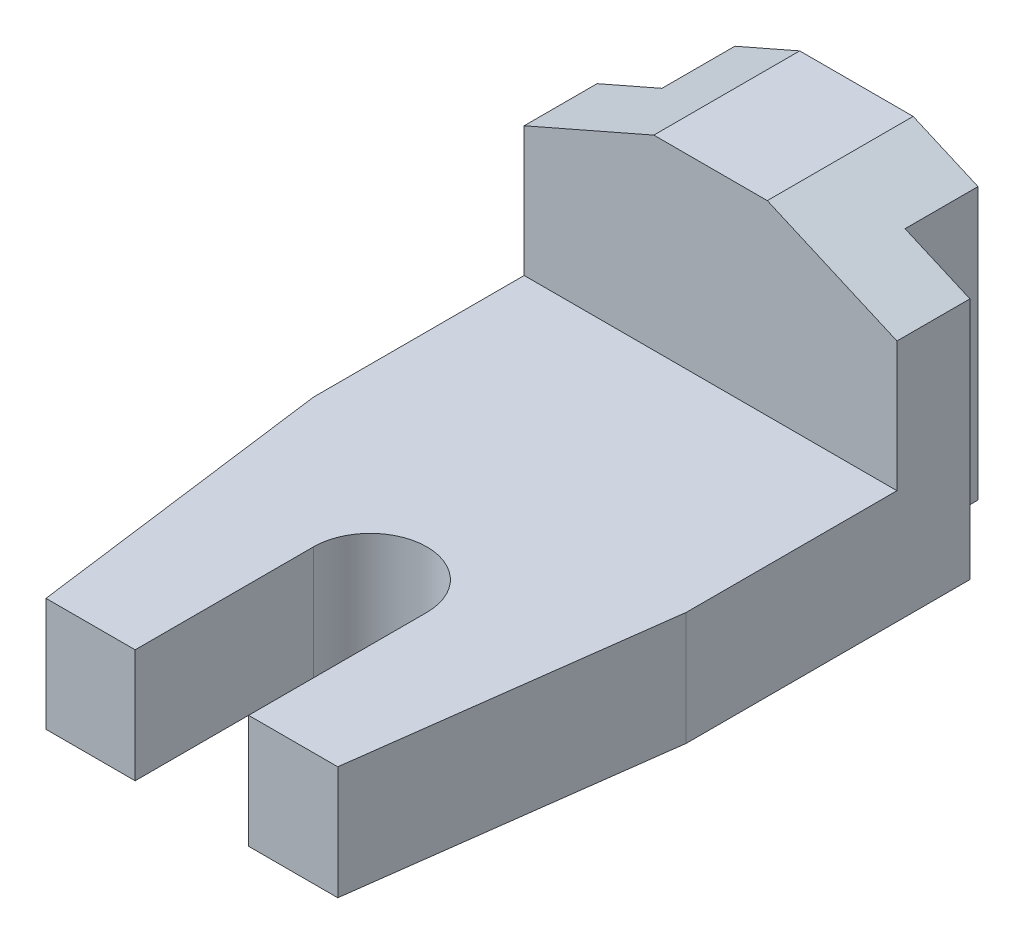
ISO-10303-21;
HEADER;
FILE_DESCRIPTION(('STEP AP214'),'2;1');
FILE_NAME('part.step','',(''),(''),'','','');
FILE_SCHEMA(('AUTOMOTIVE_DESIGN { 1 0 10303 214 1 1 1 1 }'));
ENDSEC;
DATA;
#1=APPLICATION_CONTEXT('core data for automotive mechanical design processes');
#2=APPLICATION_PROTOCOL_DEFINITION('international standard','automotive_design',2000,#1);
#3=PRODUCT_CONTEXT('',#1,'mechanical');
#4=PRODUCT('Part','Part','',(#3));
#5=PRODUCT_RELATED_PRODUCT_CATEGORY('part','',(#4));
#6=PRODUCT_DEFINITION_FORMATION('','',#4);
#7=PRODUCT_DEFINITION_CONTEXT('part definition',#1,'design');
#8=PRODUCT_DEFINITION('design','',#6,#7);
#9=PRODUCT_DEFINITION_SHAPE('','',#8);
#10=(LENGTH_UNIT() NAMED_UNIT(*) SI_UNIT(.MILLI.,.METRE.));
#11=(NAMED_UNIT(*) PLANE_ANGLE_UNIT() SI_UNIT($,.RADIAN.));
#12=(NAMED_UNIT(*) SI_UNIT($,.STERADIAN.) SOLID_ANGLE_UNIT());
#13=UNCERTAINTY_MEASURE_WITH_UNIT(LENGTH_MEASURE(1.E-05),#10,'distance_accuracy_value','');
#14=(GEOMETRIC_REPRESENTATION_CONTEXT(3) GLOBAL_UNCERTAINTY_ASSIGNED_CONTEXT((#13)) GLOBAL_UNIT_ASSIGNED_CONTEXT((#10,
#11,#12)) REPRESENTATION_CONTEXT('',''));
#15=CARTESIAN_POINT('',(0.,0.,0.));
#16=DIRECTION('',(0.,0.,1.));
#17=DIRECTION('',(1.,0.,0.));
#18=AXIS2_PLACEMENT_3D('',#15,#16,#17);
#19=CARTESIAN_POINT('',(-23.,-15.,18.));
#20=DIRECTION('',(1.,0.,0.));
#21=DIRECTION('',(0.,0.,-1.));
#22=AXIS2_PLACEMENT_3D('',#19,#20,#21);
#23=PLANE('',#22);
#24=DIRECTION('',(0.,-1.,0.));
#25=VECTOR('',#24,1.);
#26=CARTESIAN_POINT('',(-23.,22.,9.));
#27=LINE('',#26,#25);
#28=CARTESIAN_POINT('',(-23.,15.,9.));
#29=VERTEX_POINT('',#28);
#30=CARTESIAN_POINT('',(-23.,-15.,9.));
#31=VERTEX_POINT('',#30);
#32=EDGE_CURVE('E332',#29,#31,#27,.T.);
#33=ORIENTED_EDGE('',*,*,#32,.T.);
#34=DIRECTION('',(0.,0.,-1.));
#35=VECTOR('',#34,1.);
#36=CARTESIAN_POINT('',(-23.,-15.,18.));
#37=LINE('',#36,#35);
#38=CARTESIAN_POINT('',(-23.,-15.,44.));
#39=VERTEX_POINT('',#38);
#40=EDGE_CURVE('E207',#39,#31,#37,.T.);
#41=ORIENTED_EDGE('',*,*,#40,.F.);
#42=DIRECTION('',(0.,-1.,0.));
#43=VECTOR('',#42,1.);
#44=CARTESIAN_POINT('',(-23.,-0.999999999999997,44.));
#45=LINE('',#44,#43);
#46=CARTESIAN_POINT('',(-23.,-0.999999999999997,44.));
#47=VERTEX_POINT('',#46);
#48=EDGE_CURVE('E177',#47,#39,#45,.T.);
#49=ORIENTED_EDGE('',*,*,#48,.F.);
#50=DIRECTION('',(0.,0.,-1.));
#51=VECTOR('',#50,1.);
#52=CARTESIAN_POINT('',(-23.,-0.999999999999997,18.));
#53=LINE('',#52,#51);
#54=CARTESIAN_POINT('',(-23.,-0.999999999999997,18.));
#55=VERTEX_POINT('',#54);
#56=EDGE_CURVE('E270',#47,#55,#53,.T.);
#57=ORIENTED_EDGE('',*,*,#56,.T.);
#58=DIRECTION('',(0.,-1.,0.));
#59=VECTOR('',#58,1.);
#60=CARTESIAN_POINT('',(-23.,-15.,18.));
#61=LINE('',#60,#59);
#62=CARTESIAN_POINT('',(-23.,15.,18.));
#63=VERTEX_POINT('',#62);
#64=EDGE_CURVE('E193',#63,#55,#61,.T.);
#65=ORIENTED_EDGE('',*,*,#64,.F.);
#66=DIRECTION('',(0.,0.,-1.));
#67=VECTOR('',#66,1.);
#68=CARTESIAN_POINT('',(-23.,15.,18.));
#69=LINE('',#68,#67);
#70=EDGE_CURVE('E192',#63,#29,#69,.T.);
#71=ORIENTED_EDGE('',*,*,#70,.T.);
#72=EDGE_LOOP('',(#33,#41,#49,#57,#65,#71));
#73=FACE_BOUND('',#72,.T.);
#74=ADVANCED_FACE('F39',(#73),#23,.F.);
#75=CARTESIAN_POINT('',(23.,-15.,18.));
#76=DIRECTION('',(0.,1.,0.));
#77=DIRECTION('',(-1.,0.,0.));
#78=AXIS2_PLACEMENT_3D('',#75,#76,#77);
#79=PLANE('',#78);
#80=DIRECTION('',(1.,0.,0.));
#81=VECTOR('',#80,1.);
#82=CARTESIAN_POINT('',(-23.,-15.,9.));
#83=LINE('',#82,#81);
#84=CARTESIAN_POINT('',(-15.,-15.,9.));
#85=VERTEX_POINT('',#84);
#86=EDGE_CURVE('E174',#31,#85,#83,.T.);
#87=ORIENTED_EDGE('',*,*,#86,.T.);
#88=DIRECTION('',(0.,0.,-1.));
#89=VECTOR('',#88,1.);
#90=CARTESIAN_POINT('',(-15.,-15.,0.));
#91=LINE('',#90,#89);
#92=CARTESIAN_POINT('',(-15.,-15.,0.));
#93=VERTEX_POINT('',#92);
#94=EDGE_CURVE('E163',#85,#93,#91,.T.);
#95=ORIENTED_EDGE('',*,*,#94,.T.);
#96=DIRECTION('',(1.,0.,0.));
#97=VECTOR('',#96,1.);
#98=CARTESIAN_POINT('',(23.,-15.,0.));
#99=LINE('',#98,#97);
#100=CARTESIAN_POINT('',(15.,-15.,0.));
#101=VERTEX_POINT('',#100);
#102=EDGE_CURVE('E63',#93,#101,#99,.T.);
#103=ORIENTED_EDGE('',*,*,#102,.T.);
#104=DIRECTION('',(0.,0.,-1.));
#105=VECTOR('',#104,1.);
#106=CARTESIAN_POINT('',(15.,-15.,0.));
#107=LINE('',#106,#105);
#108=CARTESIAN_POINT('',(15.,-15.,9.));
#109=VERTEX_POINT('',#108);
#110=EDGE_CURVE('E231',#109,#101,#107,.T.);
#111=ORIENTED_EDGE('',*,*,#110,.F.);
#112=DIRECTION('',(-1.,0.,0.));
#113=VECTOR('',#112,1.);
#114=CARTESIAN_POINT('',(23.,-15.,9.));
#115=LINE('',#114,#113);
#116=CARTESIAN_POINT('',(23.,-15.,9.));
#117=VERTEX_POINT('',#116);
#118=EDGE_CURVE('E232',#117,#109,#115,.T.);
#119=ORIENTED_EDGE('',*,*,#118,.F.);
#120=DIRECTION('',(0.,0.,-1.));
#121=VECTOR('',#120,1.);
#122=CARTESIAN_POINT('',(23.,-15.,18.));
#123=LINE('',#122,#121);
#124=CARTESIAN_POINT('',(23.,-15.,44.));
#125=VERTEX_POINT('',#124);
#126=EDGE_CURVE('E206',#125,#117,#123,.T.);
#127=ORIENTED_EDGE('',*,*,#126,.F.);
#128=DIRECTION('',(-0.130454512571387,0.,0.991454295542544));
#129=VECTOR('',#128,1.);
#130=CARTESIAN_POINT('',(23.,-15.,44.));
#131=LINE('',#130,#129);
#132=CARTESIAN_POINT('',(18.,-15.,82.));
#133=VERTEX_POINT('',#132);
#134=EDGE_CURVE('E236',#125,#133,#131,.T.);
#135=ORIENTED_EDGE('',*,*,#134,.T.);
#136=DIRECTION('',(-1.,0.,0.));
#137=VECTOR('',#136,1.);
#138=CARTESIAN_POINT('',(18.,-15.,82.));
#139=LINE('',#138,#137);
#140=CARTESIAN_POINT('',(6.99999999999999,-15.,82.));
#141=VERTEX_POINT('',#140);
#142=EDGE_CURVE('E272',#133,#141,#139,.T.);
#143=ORIENTED_EDGE('',*,*,#142,.T.);
#144=DIRECTION('',(0.,0.,-1.));
#145=VECTOR('',#144,1.);
#146=CARTESIAN_POINT('',(6.99999999999999,-15.,82.));
#147=LINE('',#146,#145);
#148=CARTESIAN_POINT('',(6.99999999999999,-15.,60.));
#149=VERTEX_POINT('',#148);
#150=EDGE_CURVE('E277',#141,#149,#147,.T.);
#151=ORIENTED_EDGE('',*,*,#150,.T.);
#152=CARTESIAN_POINT('',(0.,-15.,60.));
#153=DIRECTION('',(0.,1.,0.));
#154=DIRECTION('',(1.,0.,0.));
#155=AXIS2_PLACEMENT_3D('',#152,#153,#154);
#156=CIRCLE('',#155,7.);
#157=CARTESIAN_POINT('',(-6.99999999999999,-15.,60.));
#158=VERTEX_POINT('',#157);
#159=EDGE_CURVE('E276',#149,#158,#156,.T.);
#160=ORIENTED_EDGE('',*,*,#159,.T.);
#161=DIRECTION('',(0.,0.,1.));
#162=VECTOR('',#161,1.);
#163=CARTESIAN_POINT('',(-7.00000000000001,-15.,82.));
#164=LINE('',#163,#162);
#165=CARTESIAN_POINT('',(-7.00000000000001,-15.,82.));
#166=VERTEX_POINT('',#165);
#167=EDGE_CURVE('E284',#158,#166,#164,.T.);
#168=ORIENTED_EDGE('',*,*,#167,.T.);
#169=DIRECTION('',(-1.,0.,0.));
#170=VECTOR('',#169,1.);
#171=CARTESIAN_POINT('',(-18.,-15.,82.));
#172=LINE('',#171,#170);
#173=CARTESIAN_POINT('',(-18.,-15.,82.));
#174=VERTEX_POINT('',#173);
#175=EDGE_CURVE('E281',#166,#174,#172,.T.);
#176=ORIENTED_EDGE('',*,*,#175,.T.);
#177=DIRECTION('',(-0.130454512571387,0.,-0.991454295542544));
#178=VECTOR('',#177,1.);
#179=CARTESIAN_POINT('',(-23.,-15.,44.));
#180=LINE('',#179,#178);
#181=EDGE_CURVE('E242',#174,#39,#180,.T.);
#182=ORIENTED_EDGE('',*,*,#181,.T.);
#183=ORIENTED_EDGE('',*,*,#40,.T.);
#184=EDGE_LOOP('',(#87,#95,#103,#111,#119,#127,#135,#143,#151,#160,#168,#176,#182,#183));
#185=FACE_BOUND('',#184,.T.);
#186=ADVANCED_FACE('F168',(#185),#79,.F.);
#187=CARTESIAN_POINT('',(-23.,15.,18.));
#188=DIRECTION('',(0.400818834019708,-0.916157334902189,0.));
#189=DIRECTION('',(0.916157334902189,0.400818834019708,0.));
#190=AXIS2_PLACEMENT_3D('',#187,#188,#189);
#191=PLANE('',#190);
#192=DIRECTION('',(0.916157334902189,0.400818834019708,0.));
#193=VECTOR('',#192,1.);
#194=CARTESIAN_POINT('',(-23.,15.,9.));
#195=LINE('',#194,#193);
#196=CARTESIAN_POINT('',(-15.,18.5,9.));
#197=VERTEX_POINT('',#196);
#198=EDGE_CURVE('E11',#29,#197,#195,.T.);
#199=ORIENTED_EDGE('',*,*,#198,.F.);
#200=ORIENTED_EDGE('',*,*,#70,.F.);
#201=DIRECTION('',(-0.916157334902189,-0.400818834019708,0.));
#202=VECTOR('',#201,1.);
#203=CARTESIAN_POINT('',(-23.,15.,18.));
#204=LINE('',#203,#202);
#205=CARTESIAN_POINT('',(-7.,22.,18.));
#206=VERTEX_POINT('',#205);
#207=EDGE_CURVE('E189',#206,#63,#204,.T.);
#208=ORIENTED_EDGE('',*,*,#207,.F.);
#209=DIRECTION('',(0.,0.,-1.));
#210=VECTOR('',#209,1.);
#211=CARTESIAN_POINT('',(-7.,22.,18.));
#212=LINE('',#211,#210);
#213=CARTESIAN_POINT('',(-7.,22.,0.));
#214=VERTEX_POINT('',#213);
#215=EDGE_CURVE('E197',#206,#214,#212,.T.);
#216=ORIENTED_EDGE('',*,*,#215,.T.);
#217=DIRECTION('',(-0.916157334902189,-0.400818834019708,0.));
#218=VECTOR('',#217,1.);
#219=CARTESIAN_POINT('',(-23.,15.,0.));
#220=LINE('',#219,#218);
#221=CARTESIAN_POINT('',(-15.,18.5,0.));
#222=VERTEX_POINT('',#221);
#223=EDGE_CURVE('E191',#214,#222,#220,.T.);
#224=ORIENTED_EDGE('',*,*,#223,.T.);
#225=DIRECTION('',(0.,0.,-1.));
#226=VECTOR('',#225,1.);
#227=CARTESIAN_POINT('',(-15.,18.5,18.));
#228=LINE('',#227,#226);
#229=EDGE_CURVE('E52',#197,#222,#228,.T.);
#230=ORIENTED_EDGE('',*,*,#229,.F.);
#231=EDGE_LOOP('',(#199,#200,#208,#216,#224,#230));
#232=FACE_BOUND('',#231,.T.);
#233=ADVANCED_FACE('F320',(#232),#191,.F.);
#234=CARTESIAN_POINT('',(0.,0.,0.));
#235=DIRECTION('',(0.,0.,-1.));
#236=DIRECTION('',(-1.,0.,0.));
#237=AXIS2_PLACEMENT_3D('',#234,#235,#236);
#238=PLANE('',#237);
#239=ORIENTED_EDGE('',*,*,#102,.F.);
#240=DIRECTION('',(0.,1.,0.));
#241=VECTOR('',#240,1.);
#242=CARTESIAN_POINT('',(-15.,0.,0.));
#243=LINE('',#242,#241);
#244=EDGE_CURVE('E46',#93,#222,#243,.T.);
#245=ORIENTED_EDGE('',*,*,#244,.T.);
#246=ORIENTED_EDGE('',*,*,#223,.F.);
#247=DIRECTION('',(-1.,0.,0.));
#248=VECTOR('',#247,1.);
#249=CARTESIAN_POINT('',(-7.,22.,0.));
#250=LINE('',#249,#248);
#251=CARTESIAN_POINT('',(7.,22.,0.));
#252=VERTEX_POINT('',#251);
#253=EDGE_CURVE('E182',#252,#214,#250,.T.);
#254=ORIENTED_EDGE('',*,*,#253,.F.);
#255=DIRECTION('',(-0.916157334902189,0.400818834019708,0.));
#256=VECTOR('',#255,1.);
#257=CARTESIAN_POINT('',(7.,22.,0.));
#258=LINE('',#257,#256);
#259=CARTESIAN_POINT('',(15.,18.5,0.));
#260=VERTEX_POINT('',#259);
#261=EDGE_CURVE('E178',#260,#252,#258,.T.);
#262=ORIENTED_EDGE('',*,*,#261,.F.);
#263=DIRECTION('',(0.,1.,0.));
#264=VECTOR('',#263,1.);
#265=CARTESIAN_POINT('',(15.,0.,0.));
#266=LINE('',#265,#264);
#267=EDGE_CURVE('E180',#101,#260,#266,.T.);
#268=ORIENTED_EDGE('',*,*,#267,.F.);
#269=EDGE_LOOP('',(#239,#245,#246,#254,#262,#268));
#270=FACE_BOUND('',#269,.T.);
#271=ADVANCED_FACE('F171',(#270),#238,.T.);
#272=CARTESIAN_POINT('',(23.,-15.,18.));
#273=DIRECTION('',(-1.,0.,0.));
#274=DIRECTION('',(0.,0.,1.));
#275=AXIS2_PLACEMENT_3D('',#272,#273,#274);
#276=PLANE('',#275);
#277=ORIENTED_EDGE('',*,*,#126,.T.);
#278=DIRECTION('',(0.,-1.,0.));
#279=VECTOR('',#278,1.);
#280=CARTESIAN_POINT('',(23.,22.,9.));
#281=LINE('',#280,#279);
#282=CARTESIAN_POINT('',(23.,15.,9.));
#283=VERTEX_POINT('',#282);
#284=EDGE_CURVE('E221',#283,#117,#281,.T.);
#285=ORIENTED_EDGE('',*,*,#284,.F.);
#286=DIRECTION('',(0.,0.,-1.));
#287=VECTOR('',#286,1.);
#288=CARTESIAN_POINT('',(23.,15.,18.));
#289=LINE('',#288,#287);
#290=CARTESIAN_POINT('',(23.,15.,18.));
#291=VERTEX_POINT('',#290);
#292=EDGE_CURVE('E201',#291,#283,#289,.T.);
#293=ORIENTED_EDGE('',*,*,#292,.F.);
#294=DIRECTION('',(0.,1.,0.));
#295=VECTOR('',#294,1.);
#296=CARTESIAN_POINT('',(23.,-15.,18.));
#297=LINE('',#296,#295);
#298=CARTESIAN_POINT('',(23.,-0.999999999999996,18.));
#299=VERTEX_POINT('',#298);
#300=EDGE_CURVE('E302',#299,#291,#297,.T.);
#301=ORIENTED_EDGE('',*,*,#300,.F.);
#302=DIRECTION('',(0.,0.,1.));
#303=VECTOR('',#302,1.);
#304=CARTESIAN_POINT('',(23.,-0.999999999999994,18.));
#305=LINE('',#304,#303);
#306=CARTESIAN_POINT('',(23.,-0.999999999999994,44.));
#307=VERTEX_POINT('',#306);
#308=EDGE_CURVE('E244',#299,#307,#305,.T.);
#309=ORIENTED_EDGE('',*,*,#308,.T.);
#310=DIRECTION('',(0.,-1.,0.));
#311=VECTOR('',#310,1.);
#312=CARTESIAN_POINT('',(23.,-0.999999999999994,44.));
#313=LINE('',#312,#311);
#314=EDGE_CURVE('E269',#307,#125,#313,.T.);
#315=ORIENTED_EDGE('',*,*,#314,.T.);
#316=EDGE_LOOP('',(#277,#285,#293,#301,#309,#315));
#317=FACE_BOUND('',#316,.T.);
#318=ADVANCED_FACE('F227',(#317),#276,.F.);
#319=CARTESIAN_POINT('',(7.,22.,18.));
#320=DIRECTION('',(-0.400818834019708,-0.916157334902189,0.));
#321=DIRECTION('',(0.916157334902189,-0.400818834019708,0.));
#322=AXIS2_PLACEMENT_3D('',#319,#320,#321);
#323=PLANE('',#322);
#324=DIRECTION('',(-0.916157334902189,0.400818834019708,0.));
#325=VECTOR('',#324,1.);
#326=CARTESIAN_POINT('',(7.,22.,9.));
#327=LINE('',#326,#325);
#328=CARTESIAN_POINT('',(15.,18.5,9.));
#329=VERTEX_POINT('',#328);
#330=EDGE_CURVE('E166',#283,#329,#327,.T.);
#331=ORIENTED_EDGE('',*,*,#330,.T.);
#332=DIRECTION('',(0.,0.,-1.));
#333=VECTOR('',#332,1.);
#334=CARTESIAN_POINT('',(15.,18.5,18.));
#335=LINE('',#334,#333);
#336=EDGE_CURVE('E216',#329,#260,#335,.T.);
#337=ORIENTED_EDGE('',*,*,#336,.T.);
#338=ORIENTED_EDGE('',*,*,#261,.T.);
#339=DIRECTION('',(0.,0.,-1.));
#340=VECTOR('',#339,1.);
#341=CARTESIAN_POINT('',(7.,22.,18.));
#342=LINE('',#341,#340);
#343=CARTESIAN_POINT('',(7.,22.,18.));
#344=VERTEX_POINT('',#343);
#345=EDGE_CURVE('E199',#344,#252,#342,.T.);
#346=ORIENTED_EDGE('',*,*,#345,.F.);
#347=DIRECTION('',(-0.916157334902189,0.400818834019708,0.));
#348=VECTOR('',#347,1.);
#349=CARTESIAN_POINT('',(7.,22.,18.));
#350=LINE('',#349,#348);
#351=EDGE_CURVE('E308',#291,#344,#350,.T.);
#352=ORIENTED_EDGE('',*,*,#351,.F.);
#353=ORIENTED_EDGE('',*,*,#292,.T.);
#354=EDGE_LOOP('',(#331,#337,#338,#346,#352,#353));
#355=FACE_BOUND('',#354,.T.);
#356=ADVANCED_FACE('F214',(#355),#323,.F.);
#357=CARTESIAN_POINT('',(-7.,22.,18.));
#358=DIRECTION('',(0.,-1.,0.));
#359=DIRECTION('',(0.,0.,-1.));
#360=AXIS2_PLACEMENT_3D('',#357,#358,#359);
#361=PLANE('',#360);
#362=ORIENTED_EDGE('',*,*,#253,.T.);
#363=ORIENTED_EDGE('',*,*,#215,.F.);
#364=DIRECTION('',(-1.,0.,0.));
#365=VECTOR('',#364,1.);
#366=CARTESIAN_POINT('',(-7.,22.,18.));
#367=LINE('',#366,#365);
#368=EDGE_CURVE('E307',#344,#206,#367,.T.);
#369=ORIENTED_EDGE('',*,*,#368,.F.);
#370=ORIENTED_EDGE('',*,*,#345,.T.);
#371=EDGE_LOOP('',(#362,#363,#369,#370));
#372=FACE_BOUND('',#371,.T.);
#373=ADVANCED_FACE('F381',(#372),#361,.F.);
#374=CARTESIAN_POINT('',(0.,0.,18.));
#375=DIRECTION('',(0.,0.,-1.));
#376=DIRECTION('',(-1.,0.,0.));
#377=AXIS2_PLACEMENT_3D('',#374,#375,#376);
#378=PLANE('',#377);
#379=ORIENTED_EDGE('',*,*,#64,.T.);
#380=DIRECTION('',(1.,0.,0.));
#381=VECTOR('',#380,1.);
#382=CARTESIAN_POINT('',(23.,-0.999999999999994,18.));
#383=LINE('',#382,#381);
#384=EDGE_CURVE('E239',#55,#299,#383,.T.);
#385=ORIENTED_EDGE('',*,*,#384,.T.);
#386=ORIENTED_EDGE('',*,*,#300,.T.);
#387=ORIENTED_EDGE('',*,*,#351,.T.);
#388=ORIENTED_EDGE('',*,*,#368,.T.);
#389=ORIENTED_EDGE('',*,*,#207,.T.);
#390=EDGE_LOOP('',(#379,#385,#386,#387,#388,#389));
#391=FACE_BOUND('',#390,.T.);
#392=ADVANCED_FACE('F311',(#391),#378,.F.);
#393=CARTESIAN_POINT('',(-23.,-0.999999999999997,44.));
#394=DIRECTION('',(-0.991454295542544,0.,0.130454512571387));
#395=DIRECTION('',(0.130454512571387,0.,0.991454295542544));
#396=AXIS2_PLACEMENT_3D('',#393,#394,#395);
#397=PLANE('',#396);
#398=ORIENTED_EDGE('',*,*,#181,.F.);
#399=DIRECTION('',(0.,-1.,0.));
#400=VECTOR('',#399,1.);
#401=CARTESIAN_POINT('',(-18.,-0.999999999999997,82.));
#402=LINE('',#401,#400);
#403=CARTESIAN_POINT('',(-18.,-0.999999999999997,82.));
#404=VERTEX_POINT('',#403);
#405=EDGE_CURVE('E184',#404,#174,#402,.T.);
#406=ORIENTED_EDGE('',*,*,#405,.F.);
#407=DIRECTION('',(-0.130454512571387,0.,-0.991454295542544));
#408=VECTOR('',#407,1.);
#409=CARTESIAN_POINT('',(-23.,-0.999999999999997,44.));
#410=LINE('',#409,#408);
#411=EDGE_CURVE('E262',#404,#47,#410,.T.);
#412=ORIENTED_EDGE('',*,*,#411,.T.);
#413=ORIENTED_EDGE('',*,*,#48,.T.);
#414=EDGE_LOOP('',(#398,#406,#412,#413));
#415=FACE_BOUND('',#414,.T.);
#416=ADVANCED_FACE('F341',(#415),#397,.T.);
#417=CARTESIAN_POINT('',(-18.,-0.999999999999997,82.));
#418=DIRECTION('',(0.,0.,1.));
#419=DIRECTION('',(1.,0.,0.));
#420=AXIS2_PLACEMENT_3D('',#417,#418,#419);
#421=PLANE('',#420);
#422=ORIENTED_EDGE('',*,*,#175,.F.);
#423=DIRECTION('',(0.,-1.,0.));
#424=VECTOR('',#423,1.);
#425=CARTESIAN_POINT('',(-7.00000000000001,-0.999999999999996,82.));
#426=LINE('',#425,#424);
#427=CARTESIAN_POINT('',(-7.00000000000001,-0.999999999999996,82.));
#428=VERTEX_POINT('',#427);
#429=EDGE_CURVE('E292',#428,#166,#426,.T.);
#430=ORIENTED_EDGE('',*,*,#429,.F.);
#431=DIRECTION('',(-1.,0.,0.));
#432=VECTOR('',#431,1.);
#433=CARTESIAN_POINT('',(-18.,-0.999999999999997,82.));
#434=LINE('',#433,#432);
#435=EDGE_CURVE('E261',#428,#404,#434,.T.);
#436=ORIENTED_EDGE('',*,*,#435,.T.);
#437=ORIENTED_EDGE('',*,*,#405,.T.);
#438=EDGE_LOOP('',(#422,#430,#436,#437));
#439=FACE_BOUND('',#438,.T.);
#440=ADVANCED_FACE('F343',(#439),#421,.T.);
#441=CARTESIAN_POINT('',(-7.00000000000001,-0.999999999999996,82.));
#442=DIRECTION('',(1.,0.,0.));
#443=DIRECTION('',(0.,0.,-1.));
#444=AXIS2_PLACEMENT_3D('',#441,#442,#443);
#445=PLANE('',#444);
#446=ORIENTED_EDGE('',*,*,#167,.F.);
#447=DIRECTION('',(0.,-1.,0.));
#448=VECTOR('',#447,1.);
#449=CARTESIAN_POINT('',(-7.,-0.999999999999996,60.));
#450=LINE('',#449,#448);
#451=CARTESIAN_POINT('',(-7.,-0.999999999999996,60.));
#452=VERTEX_POINT('',#451);
#453=EDGE_CURVE('E291',#452,#158,#450,.T.);
#454=ORIENTED_EDGE('',*,*,#453,.F.);
#455=DIRECTION('',(0.,0.,1.));
#456=VECTOR('',#455,1.);
#457=CARTESIAN_POINT('',(-7.00000000000001,-0.999999999999996,82.));
#458=LINE('',#457,#456);
#459=EDGE_CURVE('E256',#452,#428,#458,.T.);
#460=ORIENTED_EDGE('',*,*,#459,.T.);
#461=ORIENTED_EDGE('',*,*,#429,.T.);
#462=EDGE_LOOP('',(#446,#454,#460,#461));
#463=FACE_BOUND('',#462,.T.);
#464=ADVANCED_FACE('F346',(#463),#445,.T.);
#465=CARTESIAN_POINT('',(0.,-0.999999999999996,60.));
#466=DIRECTION('',(0.,-1.,0.));
#467=DIRECTION('',(1.,0.,0.));
#468=AXIS2_PLACEMENT_3D('',#465,#466,#467);
#469=CYLINDRICAL_SURFACE('',#468,7.);
#470=ORIENTED_EDGE('',*,*,#159,.F.);
#471=DIRECTION('',(0.,-1.,0.));
#472=VECTOR('',#471,1.);
#473=CARTESIAN_POINT('',(6.99999999999999,-0.999999999999996,60.));
#474=LINE('',#473,#472);
#475=CARTESIAN_POINT('',(6.99999999999999,-0.999999999999996,60.));
#476=VERTEX_POINT('',#475);
#477=EDGE_CURVE('E293',#476,#149,#474,.T.);
#478=ORIENTED_EDGE('',*,*,#477,.F.);
#479=CARTESIAN_POINT('',(0.,-0.999999999999996,60.));
#480=DIRECTION('',(0.,1.,0.));
#481=DIRECTION('',(1.,0.,0.));
#482=AXIS2_PLACEMENT_3D('',#479,#480,#481);
#483=CIRCLE('',#482,7.);
#484=EDGE_CURVE('E254',#476,#452,#483,.T.);
#485=ORIENTED_EDGE('',*,*,#484,.T.);
#486=ORIENTED_EDGE('',*,*,#453,.T.);
#487=EDGE_LOOP('',(#470,#478,#485,#486));
#488=FACE_BOUND('',#487,.T.);
#489=ADVANCED_FACE('F353',(#488),#469,.F.);
#490=CARTESIAN_POINT('',(6.99999999999999,-0.999999999999996,82.));
#491=DIRECTION('',(-1.,0.,0.));
#492=DIRECTION('',(0.,-1.,0.));
#493=AXIS2_PLACEMENT_3D('',#490,#491,#492);
#494=PLANE('',#493);
#495=ORIENTED_EDGE('',*,*,#150,.F.);
#496=DIRECTION('',(0.,-1.,0.));
#497=VECTOR('',#496,1.);
#498=CARTESIAN_POINT('',(6.99999999999999,-0.999999999999996,82.));
#499=LINE('',#498,#497);
#500=CARTESIAN_POINT('',(6.99999999999999,-0.999999999999996,82.));
#501=VERTEX_POINT('',#500);
#502=EDGE_CURVE('E299',#501,#141,#499,.T.);
#503=ORIENTED_EDGE('',*,*,#502,.F.);
#504=DIRECTION('',(0.,0.,-1.));
#505=VECTOR('',#504,1.);
#506=CARTESIAN_POINT('',(6.99999999999999,-0.999999999999996,82.));
#507=LINE('',#506,#505);
#508=EDGE_CURVE('E252',#501,#476,#507,.T.);
#509=ORIENTED_EDGE('',*,*,#508,.T.);
#510=ORIENTED_EDGE('',*,*,#477,.T.);
#511=EDGE_LOOP('',(#495,#503,#509,#510));
#512=FACE_BOUND('',#511,.T.);
#513=ADVANCED_FACE('F356',(#512),#494,.T.);
#514=CARTESIAN_POINT('',(18.,-0.999999999999994,82.));
#515=DIRECTION('',(0.,0.,1.));
#516=DIRECTION('',(1.,0.,0.));
#517=AXIS2_PLACEMENT_3D('',#514,#515,#516);
#518=PLANE('',#517);
#519=ORIENTED_EDGE('',*,*,#142,.F.);
#520=DIRECTION('',(0.,-1.,0.));
#521=VECTOR('',#520,1.);
#522=CARTESIAN_POINT('',(18.,-0.999999999999994,82.));
#523=LINE('',#522,#521);
#524=CARTESIAN_POINT('',(18.,-0.999999999999994,82.));
#525=VERTEX_POINT('',#524);
#526=EDGE_CURVE('E300',#525,#133,#523,.T.);
#527=ORIENTED_EDGE('',*,*,#526,.F.);
#528=DIRECTION('',(-1.,0.,0.));
#529=VECTOR('',#528,1.);
#530=CARTESIAN_POINT('',(18.,-0.999999999999994,82.));
#531=LINE('',#530,#529);
#532=EDGE_CURVE('E247',#525,#501,#531,.T.);
#533=ORIENTED_EDGE('',*,*,#532,.T.);
#534=ORIENTED_EDGE('',*,*,#502,.T.);
#535=EDGE_LOOP('',(#519,#527,#533,#534));
#536=FACE_BOUND('',#535,.T.);
#537=ADVANCED_FACE('F358',(#536),#518,.T.);
#538=CARTESIAN_POINT('',(23.,-0.999999999999994,44.));
#539=DIRECTION('',(0.991454295542544,0.,0.130454512571387));
#540=DIRECTION('',(0.130454512571387,0.,-0.991454295542544));
#541=AXIS2_PLACEMENT_3D('',#538,#539,#540);
#542=PLANE('',#541);
#543=ORIENTED_EDGE('',*,*,#134,.F.);
#544=ORIENTED_EDGE('',*,*,#314,.F.);
#545=DIRECTION('',(-0.130454512571387,0.,0.991454295542544));
#546=VECTOR('',#545,1.);
#547=CARTESIAN_POINT('',(23.,-0.999999999999994,44.));
#548=LINE('',#547,#546);
#549=EDGE_CURVE('E246',#307,#525,#548,.T.);
#550=ORIENTED_EDGE('',*,*,#549,.T.);
#551=ORIENTED_EDGE('',*,*,#526,.T.);
#552=EDGE_LOOP('',(#543,#544,#550,#551));
#553=FACE_BOUND('',#552,.T.);
#554=ADVANCED_FACE('F327',(#553),#542,.T.);
#555=CARTESIAN_POINT('',(0.,-0.999999999999996,60.));
#556=DIRECTION('',(0.,-1.,0.));
#557=DIRECTION('',(1.,0.,0.));
#558=AXIS2_PLACEMENT_3D('',#555,#556,#557);
#559=PLANE('',#558);
#560=ORIENTED_EDGE('',*,*,#384,.F.);
#561=ORIENTED_EDGE('',*,*,#56,.F.);
#562=ORIENTED_EDGE('',*,*,#411,.F.);
#563=ORIENTED_EDGE('',*,*,#435,.F.);
#564=ORIENTED_EDGE('',*,*,#459,.F.);
#565=ORIENTED_EDGE('',*,*,#484,.F.);
#566=ORIENTED_EDGE('',*,*,#508,.F.);
#567=ORIENTED_EDGE('',*,*,#532,.F.);
#568=ORIENTED_EDGE('',*,*,#549,.F.);
#569=ORIENTED_EDGE('',*,*,#308,.F.);
#570=EDGE_LOOP('',(#560,#561,#562,#563,#564,#565,#566,#567,#568,#569));
#571=FACE_BOUND('',#570,.T.);
#572=ADVANCED_FACE('F323',(#571),#559,.F.);
#573=CARTESIAN_POINT('',(23.,22.,9.));
#574=DIRECTION('',(0.,0.,1.));
#575=DIRECTION('',(1.,0.,0.));
#576=AXIS2_PLACEMENT_3D('',#573,#574,#575);
#577=PLANE('',#576);
#578=ORIENTED_EDGE('',*,*,#284,.T.);
#579=ORIENTED_EDGE('',*,*,#118,.T.);
#580=DIRECTION('',(0.,-1.,0.));
#581=VECTOR('',#580,1.);
#582=CARTESIAN_POINT('',(15.,22.,9.));
#583=LINE('',#582,#581);
#584=EDGE_CURVE('E228',#329,#109,#583,.T.);
#585=ORIENTED_EDGE('',*,*,#584,.F.);
#586=ORIENTED_EDGE('',*,*,#330,.F.);
#587=EDGE_LOOP('',(#578,#579,#585,#586));
#588=FACE_BOUND('',#587,.T.);
#589=ADVANCED_FACE('F225',(#588),#577,.F.);
#590=CARTESIAN_POINT('',(15.,22.,0.));
#591=DIRECTION('',(-1.,0.,0.));
#592=DIRECTION('',(0.,-1.,0.));
#593=AXIS2_PLACEMENT_3D('',#590,#591,#592);
#594=PLANE('',#593);
#595=ORIENTED_EDGE('',*,*,#584,.T.);
#596=ORIENTED_EDGE('',*,*,#110,.T.);
#597=ORIENTED_EDGE('',*,*,#267,.T.);
#598=ORIENTED_EDGE('',*,*,#336,.F.);
#599=EDGE_LOOP('',(#595,#596,#597,#598));
#600=FACE_BOUND('',#599,.T.);
#601=ADVANCED_FACE('F437',(#600),#594,.F.);
#602=CARTESIAN_POINT('',(-23.,22.,9.));
#603=DIRECTION('',(0.,0.,-1.));
#604=DIRECTION('',(-1.,0.,0.));
#605=AXIS2_PLACEMENT_3D('',#602,#603,#604);
#606=PLANE('',#605);
#607=ORIENTED_EDGE('',*,*,#198,.T.);
#608=DIRECTION('',(0.,-1.,0.));
#609=VECTOR('',#608,1.);
#610=CARTESIAN_POINT('',(-15.,22.,9.));
#611=LINE('',#610,#609);
#612=EDGE_CURVE('E331',#197,#85,#611,.T.);
#613=ORIENTED_EDGE('',*,*,#612,.T.);
#614=ORIENTED_EDGE('',*,*,#86,.F.);
#615=ORIENTED_EDGE('',*,*,#32,.F.);
#616=EDGE_LOOP('',(#607,#613,#614,#615));
#617=FACE_BOUND('',#616,.T.);
#618=ADVANCED_FACE('F443',(#617),#606,.T.);
#619=CARTESIAN_POINT('',(-15.,22.,0.));
#620=DIRECTION('',(-1.,0.,0.));
#621=DIRECTION('',(0.,-1.,0.));
#622=AXIS2_PLACEMENT_3D('',#619,#620,#621);
#623=PLANE('',#622);
#624=ORIENTED_EDGE('',*,*,#229,.T.);
#625=ORIENTED_EDGE('',*,*,#244,.F.);
#626=ORIENTED_EDGE('',*,*,#94,.F.);
#627=ORIENTED_EDGE('',*,*,#612,.F.);
#628=EDGE_LOOP('',(#624,#625,#626,#627));
#629=FACE_BOUND('',#628,.T.);
#630=ADVANCED_FACE('F162',(#629),#623,.T.);
#631=CLOSED_SHELL('',(#74,#186,#233,#271,#318,#356,#373,#392,#416,#440,#464,#489,#513,#537,#554,
#572,#589,#601,#618,#630));
#632=MANIFOLD_SOLID_BREP('B2',#631);
#633=ADVANCED_BREP_SHAPE_REPRESENTATION('',(#18,#632),#14);
#634=SHAPE_DEFINITION_REPRESENTATION(#9,#633);
ENDSEC;
END-ISO-10303-21;
